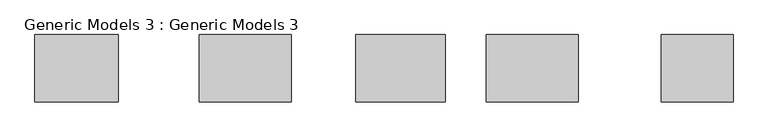
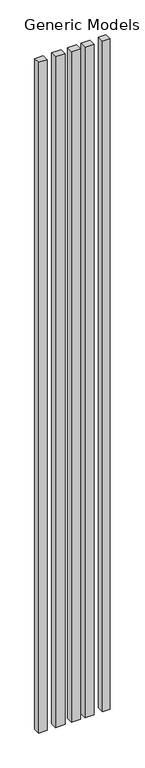
"""IFC4 building model written with IfcOpenShell, lengths in millimetres: proxy geometry, Generic Models 3 : Generic Models 3."""

from ifc_helpers import new_model, si_unit, origin, origin_with_axes, place, context, project, spatial, polyline, outline, extrude, source, transform, mapped, element, save


def generic_models_3_generic_models_3_60b2bde9(model_context):
    return source(origin(), model_context, "Body", "SweptSolid", [
        extrude(outline(polyline([(-5332.0633123, -21515.4428796), (-5440.1530431, -21515.4428796), (-5440.1530431, -21413.8428796), (-5332.0633123, -21413.8428796), (-5332.0633123, -21515.4428796)])), origin_with_axes(), (0.0, 0.0, 1.0), 10461.8702873),
        extrude(outline(polyline([(-5565.3991668, -21515.4428796), (-5704.3617833, -21515.4428796), (-5704.3617833, -21413.8428796), (-5565.3991668, -21413.8428796), (-5565.3991668, -21515.4428796)])), origin_with_axes(), (0.0, 0.0, 1.0), 10461.8702873),
        extrude(outline(polyline([(-5766.1224677, -21515.4428796), (-5901.2342193, -21515.4428796), (-5901.2342193, -21413.8428796), (-5766.1224677, -21413.8428796), (-5766.1224677, -21515.4428796)])), origin_with_axes(), (0.0, 0.0, 1.0), 10461.8702873),
        extrude(outline(polyline([(-5998.4514718, -21515.4428796), (-6137.0397558, -21515.4428796), (-6137.0397558, -21413.8428796), (-5998.4514718, -21413.8428796), (-5998.4514718, -21515.4428796)])), origin_with_axes(), (0.0, 0.0, 1.0), 10461.8702873),
        extrude(outline(polyline([(-6259.4676893, -21515.4428796), (-6384.9144224, -21515.4428796), (-6384.9144224, -21413.8428796), (-6259.4676893, -21413.8428796), (-6259.4676893, -21515.4428796)])), origin_with_axes(), (0.0, 0.0, 1.0), 10461.8702873),
    ])


if __name__ == "__main__":
    model = new_model("IFC4")
    model_context = context("Model", 3, world=origin())
    ifc_project = project(units=[si_unit("LENGTHUNIT", "METRE", prefix="MILLI")], contexts=[model_context])
    site = spatial("IfcSite", under=ifc_project)
    building = spatial("IfcBuilding", under=site)
    placement = place(None, origin())
    generic_models_3_generic_models_3_shape = generic_models_3_generic_models_3_60b2bde9(model_context)
    element("IfcBuildingElementProxy", 1, Name="Generic Models 3 : Generic Models 3", ObjectType="Generic Models 3 : Generic Models 3", at=placement, inside=building, context=model_context, shape_type="MappedRepresentation", body=[
        mapped(generic_models_3_generic_models_3_shape, transform((0.0, 0.0, 0.0), x_axis=(1.0, 0.0, 0.0), y_axis=(0.0, 1.0, 0.0), z_axis=(0.0, 0.0, 1.0))),
    ])
    save(model, "model.ifc")
